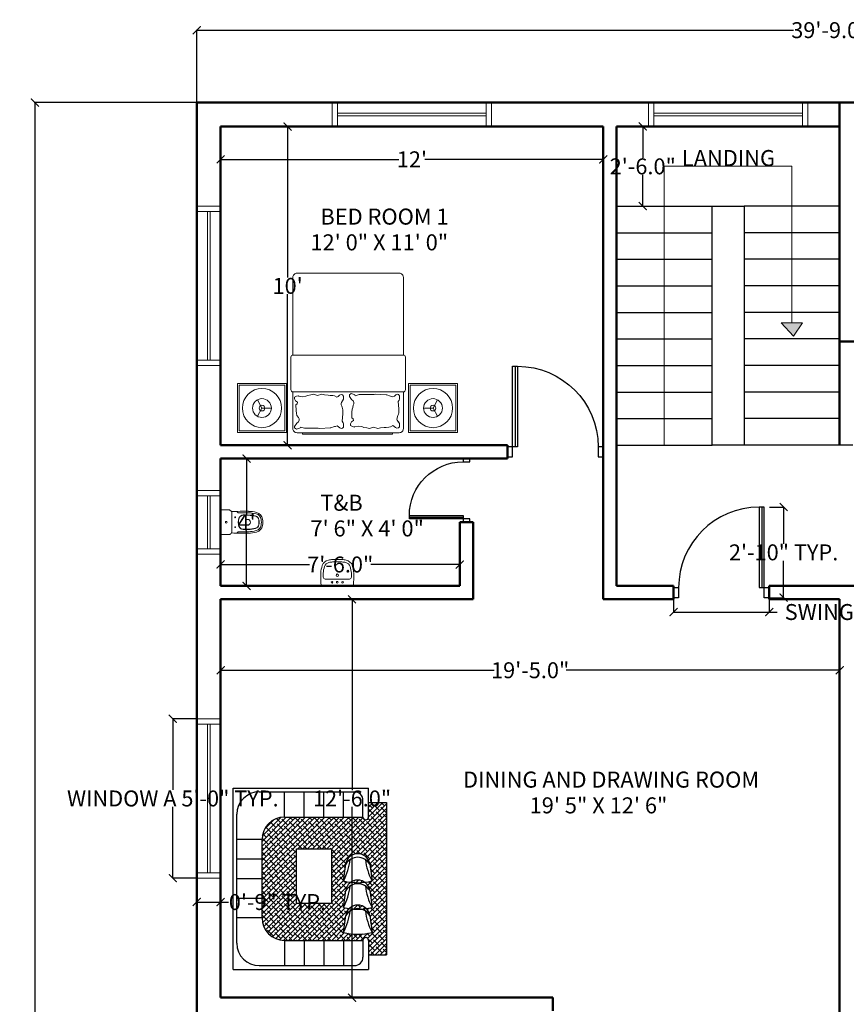
# Model space of a CAD drawing. Units: inches. Extents: x 147 to 1638, y 107 to 941.
# Tile 10 of 17: x 158 to 469, y 570 to 941. Entities that reach past the tile are written whole.
import ezdxf

# ---------------------------------------------------------------- set-up
doc = ezdxf.new("R2010")
doc.units = ezdxf.units.IN
doc.header["$MEASUREMENT"] = 0
for name, color, linetype, lineweight in [('A-ANNO-DIMS', 2, 'Continuous', 15), ('A-ANNO-SYMB', 7, 'Continuous', 18), ('A-AREA-IDEN', 7, 'Continuous', 18), ('A-Door', 150, 'Continuous', 25), ('A-FLOR-FIXT', 9, 'Continuous', 18), ('A-FLOR-STRS', 7, 'Continuous', 25), ('furniture', 50, 'Continuous', 18), ('HAT', 9, 'Continuous', 0), ('walls', 7, 'Continuous', 50), ('windows', 3, 'Continuous', 20)]:
    doc.layers.add(name, color=color, linetype=linetype, lineweight=lineweight)
for name, color, linetype in [('A-Glaz', 92, 'Continuous'), ('FUR', 42, 'Continuous'), ('NT', 1, 'Continuous'), ('Win', 152, 'Continuous')]:
    doc.layers.add(name, color=color, linetype=linetype)
doc.styles.get("Standard").update_dxf_attribs({"font": 'arial.ttf'})
doc.dimstyles.get("Standard").update_dxf_attribs({"dimtxt": 6, "dimasz": 3, "dimexe": 0.18, "dimexo": 0.0625, "dimgap": 0.09, "dimtad": 0, "dimtih": 1, "dimtoh": 1, "dimdec": 1, "dimzin": 0, "dimdsep": 46, "dimlunit": 3, "dimtxsty": 'Standard', "dimblk": 'ARCHTICK', "dimcen": 0.09, "dimadec": 0, "dimazin": 0, "dimtfac": 1, "dimtdec": 1, "dimtofl": 0, "dimtmove": 0, "dimatfit": 3, "dimfxl": 1, "dimtolj": 1, "dimtzin": 0, "dimarcsym": 0})

# ---------------------------------------------------------------- blocks, each defined once
blk = doc.blocks.new('A$C087A3AA9')
at = {"layer": 'A-Door'}
for points in [[(852.6, 94.7), (852.6, 852.6), (805.3, 852.6), (805.3, 94.7)], [(47.4, 94.7), (47.4, 0), (0, 0), (0, 94.7)], [(900, 94.7), (900, 0), (852.6, 0), (852.6, 94.7)]]:
    blk.add_lwpolyline(points, close=True, dxfattribs=at)
at = {"layer": 'A-Glaz'}
blk.add_line((828.9, 852.6), (828.9, 94.7), dxfattribs=at)
at = {"layer": 'NT'}
blk.add_arc((805.3, 94.7), 757.9, 90, 180, dxfattribs=at)
blk = doc.blocks.new('_ArchTick')
at = {"color": 0, "linetype": 'ByBlock', "const_width": 0.15}
blk.add_lwpolyline([(-0.5, -0.5), (0.5, 0.5)], dxfattribs=at)
blk = doc.blocks.new('*D3')
at = {"layer": 'A-ANNO-DIMS', "color": 0, "lineweight": -2, "transparency": 16777216}
for p, q in [((259.56, 900.72), (258.97, 900.72)), ((259.15, 900.72), (259.15, 843.87)), ((259.15, 780.72), (259.15, 837.56)), ((259.56, 780.72), (258.97, 780.72))]:
    blk.add_line(p, q, dxfattribs=at)
at = {"layer": 'Defpoints', "color": 0, "lineweight": -2, "transparency": 16777216}
for p in [(259.63, 900.72), (259.15, 780.72), (259.63, 780.72)]:
    blk.add_point(p, dxfattribs=at)
at = {"layer": 'A-ANNO-DIMS', "color": 0, "lineweight": -2, "transparency": 16777216, "xscale": 3, "yscale": 3, "zscale": 3}
for p, rotation in [((259.15, 900.72), 90), ((259.15, 780.72), 270)]:
    blk.add_blockref('_ArchTick', p, dxfattribs=dict(at, rotation=rotation))
at = {"layer": 'A-ANNO-DIMS', "color": 0, "transparency": 16777216, "insert": (259.15, 840.72), "char_height": 6, "attachment_point": 5}
blk.add_mtext("\\A1;10'", dxfattribs=at)
blk = doc.blocks.new('*D4')
at = {"layer": 'A-ANNO-DIMS', "color": 0, "lineweight": -2, "transparency": 16777216}
for p, q in [((233.94, 893.56), (233.94, 888.18)), ((377.94, 893.56), (377.94, 888.18)), ((233.94, 888.36), (301.05, 888.36)), ((377.94, 888.36), (310.84, 888.36))]:
    blk.add_line(p, q, dxfattribs=at)
at = {"layer": 'Defpoints', "color": 0, "lineweight": -2, "transparency": 16777216}
for p in [(233.94, 893.63), (377.94, 893.63), (377.94, 888.36)]:
    blk.add_point(p, dxfattribs=at)
at = {"layer": 'A-ANNO-DIMS', "color": 0, "lineweight": -2, "transparency": 16777216, "xscale": 3, "yscale": 3, "zscale": 3, "rotation": 180}
blk.add_blockref('_ArchTick', (233.94, 888.36), dxfattribs=at)
at = {"layer": 'A-ANNO-DIMS', "color": 0, "lineweight": -2, "transparency": 16777216, "xscale": 3, "yscale": 3, "zscale": 3}
blk.add_blockref('_ArchTick', (377.94, 888.36), dxfattribs=at)
at = {"layer": 'A-ANNO-DIMS', "color": 0, "transparency": 16777216, "insert": (305.94, 888.36), "char_height": 6, "attachment_point": 5}
blk.add_mtext("\\A1;12'", dxfattribs=at)
blk = doc.blocks.new('*D7')
at = {"layer": 'A-ANNO-DIMS', "color": 0, "lineweight": -2, "transparency": 16777216}
for p, q in [((389.98, 900.72), (393.01, 900.72)), ((392.83, 900.72), (392.83, 888.87)), ((392.83, 870.72), (392.83, 882.56)), ((389.98, 870.72), (393.01, 870.72))]:
    blk.add_line(p, q, dxfattribs=at)
at = {"layer": 'Defpoints', "color": 0, "lineweight": -2, "transparency": 16777216}
for p in [(389.92, 900.72), (389.92, 870.72), (392.83, 870.72)]:
    blk.add_point(p, dxfattribs=at)
at = {"layer": 'A-ANNO-DIMS', "color": 0, "lineweight": -2, "transparency": 16777216, "xscale": 3, "yscale": 3, "zscale": 3}
for p, rotation in [((392.83, 900.72), 90), ((392.83, 870.72), 270)]:
    blk.add_blockref('_ArchTick', p, dxfattribs=dict(at, rotation=rotation))
at = {"layer": 'A-ANNO-DIMS', "color": 0, "transparency": 16777216, "insert": (392.83, 885.72), "char_height": 6, "attachment_point": 5}
blk.add_mtext('\\A1;2\'-6.0"', dxfattribs=at)
blk = doc.blocks.new('*D8')
at = {"layer": 'A-ANNO-DIMS', "color": 0, "lineweight": -2, "transparency": 16777216}
for p, q in [((243.37, 775.72), (243.86, 775.72)), ((243.68, 775.72), (243.68, 754.81)), ((243.68, 727.72), (243.68, 748.63)), ((243.37, 727.72), (243.86, 727.72))]:
    blk.add_line(p, q, dxfattribs=at)
at = {"layer": 'Defpoints', "color": 0, "lineweight": -2, "transparency": 16777216}
for p in [(243.3, 775.72), (243.3, 727.72), (243.68, 727.72)]:
    blk.add_point(p, dxfattribs=at)
at = {"layer": 'A-ANNO-DIMS', "color": 0, "lineweight": -2, "transparency": 16777216, "xscale": 3, "yscale": 3, "zscale": 3}
for p, rotation in [((243.68, 775.72), 90), ((243.68, 727.72), 270)]:
    blk.add_blockref('_ArchTick', p, dxfattribs=dict(at, rotation=rotation))
at = {"layer": 'A-ANNO-DIMS', "color": 0, "transparency": 16777216, "insert": (243.68, 751.72), "char_height": 6, "attachment_point": 5}
blk.add_mtext("\\A1;4'", dxfattribs=at)
blk = doc.blocks.new('*D9')
at = {"layer": 'A-ANNO-DIMS', "color": 0, "lineweight": -2, "transparency": 16777216}
for p, q in [((233.94, 734.55), (233.94, 736)), ((233.94, 735.82), (267.41, 735.82)), ((323.94, 735.82), (290.48, 735.82)), ((323.94, 734.55), (323.94, 736))]:
    blk.add_line(p, q, dxfattribs=at)
at = {"layer": 'Defpoints', "color": 0, "lineweight": -2, "transparency": 16777216}
for p in [(233.94, 734.49), (323.94, 735.82), (323.94, 734.49)]:
    blk.add_point(p, dxfattribs=at)
at = {"layer": 'A-ANNO-DIMS', "color": 0, "lineweight": -2, "transparency": 16777216, "xscale": 3, "yscale": 3, "zscale": 3, "rotation": 180}
blk.add_blockref('_ArchTick', (233.94, 735.82), dxfattribs=at)
at = {"layer": 'A-ANNO-DIMS', "color": 0, "lineweight": -2, "transparency": 16777216, "xscale": 3, "yscale": 3, "zscale": 3}
blk.add_blockref('_ArchTick', (323.94, 735.82), dxfattribs=at)
at = {"layer": 'A-ANNO-DIMS', "color": 0, "transparency": 16777216, "insert": (278.94, 735.82), "char_height": 6, "attachment_point": 5}
blk.add_mtext('\\A1;7\'-6.0"', dxfattribs=at)
blk = doc.blocks.new('*D12')
at = {"layer": 'A-ANNO-DIMS', "color": 0, "lineweight": -2, "transparency": 16777216}
for p, q in [((278.02, 722.72), (283.58, 722.72)), ((283.4, 722.72), (283.4, 650.87)), ((283.4, 572.72), (283.4, 644.56)), ((278.02, 572.72), (283.58, 572.72))]:
    blk.add_line(p, q, dxfattribs=at)
at = {"layer": 'Defpoints', "color": 0, "lineweight": -2, "transparency": 16777216}
for p in [(277.96, 722.72), (277.96, 572.72), (283.4, 572.72)]:
    blk.add_point(p, dxfattribs=at)
at = {"layer": 'A-ANNO-DIMS', "color": 0, "lineweight": -2, "transparency": 16777216, "xscale": 3, "yscale": 3, "zscale": 3}
for p, rotation in [((283.4, 722.72), 90), ((283.4, 572.72), 270)]:
    blk.add_blockref('_ArchTick', p, dxfattribs=dict(at, rotation=rotation))
at = {"layer": 'A-ANNO-DIMS', "color": 0, "transparency": 16777216, "insert": (283.4, 647.72), "char_height": 6, "attachment_point": 5}
blk.add_mtext('\\A1;12\'-6.0"', dxfattribs=at)
blk = doc.blocks.new('*D13')
at = {"layer": 'A-ANNO-DIMS', "color": 0, "lineweight": -2, "transparency": 16777216}
for p, q in [((233.94, 696.06), (233.94, 696.18)), ((233.94, 696), (336.84, 696)), ((466.94, 696), (364.05, 696)), ((466.94, 696.06), (466.94, 696.18))]:
    blk.add_line(p, q, dxfattribs=at)
at = {"layer": 'Defpoints', "color": 0, "lineweight": -2, "transparency": 16777216}
for p in [(233.94, 696), (466.94, 696), (466.94, 696)]:
    blk.add_point(p, dxfattribs=at)
at = {"layer": 'A-ANNO-DIMS', "color": 0, "lineweight": -2, "transparency": 16777216, "xscale": 3, "yscale": 3, "zscale": 3, "rotation": 180}
blk.add_blockref('_ArchTick', (233.94, 696), dxfattribs=at)
at = {"layer": 'A-ANNO-DIMS', "color": 0, "lineweight": -2, "transparency": 16777216, "xscale": 3, "yscale": 3, "zscale": 3}
blk.add_blockref('_ArchTick', (466.94, 696), dxfattribs=at)
at = {"layer": 'A-ANNO-DIMS', "color": 0, "transparency": 16777216, "insert": (350.44, 696), "char_height": 6, "attachment_point": 5}
blk.add_mtext('\\A1;19\'-5.0"', dxfattribs=at)
blk = doc.blocks.new('*D69')
at = {"layer": 'A-ANNO-DIMS', "color": 0, "lineweight": -2, "transparency": 16777216}
for p, q in [((224.94, 909.78), (224.94, 937.18)), ((224.94, 937), (449.56, 937)), ((701.94, 937), (477.33, 937)), ((701.94, 909.78), (701.94, 937.18))]:
    blk.add_line(p, q, dxfattribs=at)
at = {"layer": 'Defpoints', "color": 0, "lineweight": -2, "transparency": 16777216}
for p in [(701.94, 937), (224.94, 909.72), (701.94, 909.72)]:
    blk.add_point(p, dxfattribs=at)
at = {"layer": 'A-ANNO-DIMS', "color": 0, "lineweight": -2, "transparency": 16777216, "xscale": 3, "yscale": 3, "zscale": 3, "rotation": 180}
blk.add_blockref('_ArchTick', (224.94, 937), dxfattribs=at)
at = {"layer": 'A-ANNO-DIMS', "color": 0, "lineweight": -2, "transparency": 16777216, "xscale": 3, "yscale": 3, "zscale": 3}
blk.add_blockref('_ArchTick', (701.94, 937), dxfattribs=at)
at = {"layer": 'A-ANNO-DIMS', "color": 0, "transparency": 16777216, "insert": (463.44, 937), "char_height": 6, "attachment_point": 5}
blk.add_mtext('\\A1;39\'-9.0"', dxfattribs=at)
blk = doc.blocks.new('*D70')
at = {"layer": 'A-ANNO-DIMS', "color": 0, "lineweight": -2, "transparency": 16777216}
for p, q in [((224.88, 909.72), (163.8, 909.72)), ((163.98, 909.72), (163.98, 558.87)), ((163.98, 201.72), (163.98, 552.56)), ((224.88, 201.72), (163.8, 201.72))]:
    blk.add_line(p, q, dxfattribs=at)
at = {"layer": 'Defpoints', "color": 0, "lineweight": -2, "transparency": 16777216}
for p in [(224.94, 909.72), (163.98, 201.72), (224.94, 201.72)]:
    blk.add_point(p, dxfattribs=at)
at = {"layer": 'A-ANNO-DIMS', "color": 0, "lineweight": -2, "transparency": 16777216, "xscale": 3, "yscale": 3, "zscale": 3}
for p, rotation in [((163.98, 909.72), 90), ((163.98, 201.72), 270)]:
    blk.add_blockref('_ArchTick', p, dxfattribs=dict(at, rotation=rotation))
at = {"layer": 'A-ANNO-DIMS', "color": 0, "transparency": 16777216, "insert": (163.98, 555.72), "char_height": 6, "attachment_point": 5}
blk.add_mtext("\\A1;59'", dxfattribs=at)
blk = doc.blocks.new('MAT-P14')
for p, q in [((-1.337, 1.348), (-1.337, 1.948)), ((-1.337, 1.948), (-0.737, 1.948)), ((-1.317, 1.928), (-0.757, 1.928)), ((-1.317, 1.368), (-1.317, 1.928)), ((-0.757, 1.368), (-0.757, 1.928)), ((-0.737, 1.348), (-0.737, 1.948)), ((0.625, 1.95), (-0.625, 1.95)), ((0.753, 1.348), (0.753, 1.948)), ((1.353, 1.948), (0.753, 1.948)), ((1.333, 1.928), (0.773, 1.928)), ((0.773, 1.368), (0.773, 1.928)), ((1.333, 1.368), (1.333, 1.928)), ((1.353, 1.348), (1.353, 1.948)), ((-1.037, 1.648), (-1.091, 1.749)), ((1.053, 1.648), (1.108, 1.749)), ((-1.037, 1.648), (-1.091, 1.547)), ((-1.037, 1.648), (-0.922, 1.648)), ((1.053, 1.648), (0.938, 1.648)), ((1.053, 1.648), (1.108, 1.547)), ((-1.337, 1.348), (-0.737, 1.348)), ((-1.317, 1.368), (-0.757, 1.368)), ((1.353, 1.348), (0.753, 1.348)), ((1.333, 1.368), (0.773, 1.368))]:
    blk.add_line(p, q)
for points in [[(-0.675, 1.45), (-0.675, 1.9, -0.414214), (-0.625, 1.95), (0.625, 1.95, -0.414214), (0.675, 1.9), (0.675, 1.45)], [(-0.675, 1, -0.414214), (-0.7, 1.025), (-0.7, 1.425, -0.414214), (-0.675, 1.45), (0.675, 1.45, -0.414214), (0.7, 1.425), (0.7, 1.025, -0.414214), (0.675, 1)], [(-0.625, 0, -0.414214), (-0.675, 0.05), (-0.675, 1), (0.675, 1), (0.675, 0.05, -0.414214), (0.625, 0)]]:
    blk.add_lwpolyline(points, format="xyb", close=True)
blk.add_lwpolyline([(-0.542, 1.95), (-0.542, 1.967), (0.558, 1.967), (0.558, 1.95)], close=True)
for points in [[(-0.614, 1.818), (-0.626, 1.838), (-0.626, 1.877), (-0.614, 1.891), (-0.596, 1.896), (-0.579, 1.886), (-0.563, 1.872), (-0.545, 1.863), (-0.516, 1.879), (-0.497, 1.882), (-0.465, 1.884), (-0.439, 1.887), (-0.395, 1.892), (-0.363, 1.9), (-0.309, 1.882), (-0.262, 1.897), (-0.23, 1.892), (-0.192, 1.884), (-0.166, 1.873), (-0.128, 1.868), (-0.082, 1.875), (-0.076, 1.88), (-0.052, 1.875), (-0.028, 1.861), (-0.028, 1.841), (-0.04, 1.817), (-0.064, 1.802), (-0.06, 1.781), (-0.043, 1.768), (-0.046, 1.697), (-0.05, 1.662), (-0.056, 1.64), (-0.062, 1.612), (-0.068, 1.596), (-0.068, 1.579), (-0.063, 1.56), (-0.039, 1.545), (-0.015, 1.505), (-0.015, 1.486), (-0.038, 1.471), (-0.075, 1.482), (-0.081, 1.487), (-0.087, 1.497), (-0.134, 1.481), (-0.304, 1.482), (-0.318, 1.482), (-0.335, 1.479), (-0.464, 1.488), (-0.467, 1.486), (-0.473, 1.486), (-0.517, 1.503), (-0.53, 1.505), (-0.548, 1.51), (-0.566, 1.501), (-0.581, 1.487), (-0.599, 1.477), (-0.617, 1.482), (-0.629, 1.497), (-0.629, 1.536), (-0.623, 1.55), (-0.611, 1.57), (-0.614, 1.614), (-0.615, 1.627), (-0.618, 1.644), (-0.619, 1.66), (-0.62, 1.675), (-0.62, 1.695), (-0.618, 1.707), (-0.614, 1.723), (-0.608, 1.739), (-0.604, 1.75), (-0.598, 1.771), (-0.596, 1.785), (-0.6, 1.798), (-0.614, 1.819)], [(0.069, 1.559), (0.057, 1.54), (0.057, 1.501), (0.069, 1.486), (0.087, 1.481), (0.105, 1.491), (0.121, 1.505), (0.139, 1.514), (0.168, 1.498), (0.187, 1.496), (0.219, 1.493), (0.244, 1.49), (0.289, 1.485), (0.321, 1.477), (0.374, 1.495), (0.422, 1.48), (0.454, 1.486), (0.492, 1.493), (0.517, 1.504), (0.555, 1.509), (0.602, 1.502), (0.608, 1.497), (0.632, 1.502), (0.656, 1.517), (0.656, 1.536), (0.644, 1.561), (0.62, 1.575), (0.624, 1.596), (0.641, 1.609), (0.637, 1.68), (0.633, 1.715), (0.628, 1.738), (0.606, 1.765), (0.6, 1.781), (0.6, 1.798), (0.605, 1.817), (0.629, 1.832), (0.654, 1.872), (0.654, 1.892), (0.63, 1.906), (0.593, 1.895), (0.587, 1.891), (0.581, 1.881), (0.534, 1.896), (0.379, 1.896), (0.366, 1.896), (0.348, 1.898), (0.22, 1.89), (0.216, 1.891), (0.21, 1.891), (0.167, 1.875), (0.154, 1.872), (0.136, 1.867), (0.118, 1.876), (0.102, 1.89), (0.085, 1.9), (0.067, 1.895), (0.055, 1.881), (0.055, 1.842), (0.061, 1.827), (0.073, 1.807), (0.07, 1.764), (0.069, 1.75), (0.066, 1.733), (0.065, 1.718), (0.063, 1.703), (0.063, 1.682), (0.066, 1.67), (0.07, 1.655), (0.075, 1.638), (0.079, 1.627), (0.086, 1.607), (0.087, 1.592), (0.083, 1.579), (0.07, 1.559)]]:
    blk.add_lwpolyline(points)
for centre, radius in [((-1.037, 1.648), 0.24), ((1.053, 1.648), 0.24), ((-1.037, 1.648), 0.115), ((1.053, 1.648), 0.115), ((-1.037, 1.648), 0.035), ((1.053, 1.648), 0.035)]:
    blk.add_circle(centre, radius)
blk = doc.blocks.new('2SAINDA')
at = {"color": 0, "linetype": 'ByBlock'}
for p, q in [((0, 0.188), (0, -0.188)), ((0.018, 0.2), (0.141, 0.2)), ((0.157, 0.192), (0.162, 0.188)), ((0.18, -0.164), (0.18, 0.164)), ((0.279, 0.159), (0.261, 0.176)), ((0.437, 0.047), (0.424, 0.047)), ((0.279, -0.159), (0.261, -0.176)), ((0.437, -0.047), (0.424, -0.047)), ((0.018, -0.2), (0.141, -0.2)), ((0.157, -0.192), (0.162, -0.188))]:
    blk.add_line(p, q, dxfattribs=at)
for centre, radius in [((0.09, 0), 0.0135), ((0.09, 0), 0.0135), ((0.236, 0.08), 0.0075), ((0.236, -0.08), 0.0075)]:
    blk.add_circle(centre, radius, dxfattribs=at)
for centre, radius, start, end in [((0.018, 0.18), 0.02, 90, 155.6901), ((0.141, 0.181), 0.019, 34.9372, 90), ((0.155, 0.164), 0.025, 23.3776, 73.7848), ((0.383, -5.322), 5.5, 89.2905, 92.1362), ((0.155, 0.164), 0.025, 360, 23.3776), ((0.444, -0.373), 0.55, 75.4605, 89.2905), ((0.293, 0.173), 0.02, 225, 270.9364), ((0.485, 0), 0.2, 160.016, 199.984), ((0.485, 0), 0.196, 160.016, 199.984), ((0.383, -5.322), 5.476, 89.2905, 90.9364), ((0.368, 0.043), 0.075, 90.1648, 160.016), ((0.368, 0.043), 0.071, 90.1648, 160.016), ((0.383, -5.322), 5.44, 89.2905, 90.1648), ((0.383, -5.322), 5.436, 89.2905, 90.1648), ((0.582, 0), 0.18, 170.2849, 189.7151), ((0.424, 0.027), 0.02, 90, 170.2849), ((0.437, 0), 0.047, 0, 90), ((0.437, 0), 0.047, 270, 0), ((0.444, -0.373), 0.49, 75.4605, 89.2905), ((0.444, -0.373), 0.486, 75.4605, 89.2905), ((0.444, -0.373), 0.526, 75.4605, 89.2905), ((0.549, 0.03), 0.07, 8.8162, 75.4605), ((0.549, 0.03), 0.074, 8.8162, 75.4605), ((0.549, 0.03), 0.11, 8.8162, 75.4605), ((0.549, 0.03), 0.134, 8.8162, 75.4605), ((0.355, 0), 0.266, 351.1838, 8.8162), ((0.355, 0), 0.27, 351.1838, 8.8162), ((0.355, 0), 0.306, 351.1838, 8.8162), ((0.355, 0), 0.33, 351.1838, 8.8162), ((0.293, -0.173), 0.02, 89.0636, 135), ((0.383, 5.322), 5.476, 269.0636, 270.7095), ((0.368, -0.043), 0.075, 199.984, 269.8352), ((0.368, -0.043), 0.071, 199.984, 269.8352), ((0.383, 5.322), 5.436, 269.8352, 270.7095), ((0.383, 5.322), 5.44, 269.8352, 270.7095), ((0.424, -0.027), 0.02, 189.7151, 270), ((0.444, 0.373), 0.486, 270.7095, 284.5395), ((0.444, 0.373), 0.49, 270.7095, 284.5395), ((0.444, 0.373), 0.526, 270.7095, 284.5395), ((0.444, 0.373), 0.55, 270.7095, 284.5395), ((0.549, -0.03), 0.07, 284.5395, 351.1838), ((0.549, -0.03), 0.074, 284.5395, 351.1838), ((0.549, -0.03), 0.11, 284.5395, 351.1838), ((0.549, -0.03), 0.134, 284.5395, 351.1838), ((0.018, -0.18), 0.02, 204.3099, 270), ((0.141, -0.181), 0.019, 270, 325.0628), ((0.155, -0.164), 0.025, 286.2152, 336.6224), ((0.155, -0.164), 0.025, 336.6224, 0), ((0.383, 5.322), 5.5, 267.8638, 270.7095)]:
    blk.add_arc(centre, radius, start, end, dxfattribs=at)
blk = doc.blocks.new('2SALADA2')
at = {"color": 0}
for p, q in [((-0.296, 0), (0.296, 0)), ((0.207, -0.13), (-0.207, -0.13))]:
    blk.add_line(p, q, dxfattribs=at)
for centre, radius in [((-0.1, -0.07), 0.015), ((0, -0.205), 0.023), ((0, -0.07), 0.0175), ((0.1, -0.07), 0.015)]:
    blk.add_circle(centre, radius, dxfattribs=at)
for centre, radius, start, end in [((-0.296, -0.01), 0.01, 90, 173.6262), ((0.296, -0.01), 0.01, 6.3738, 90), ((1.185, -0.175), 1.5, 173.6262, 182.693), ((1.186, -0.221), 1.454, 178.0234, 180.898), ((-0.227, -0.171), 0.04, 95.5937, 179.6995), ((-0.207, -0.38), 0.25, 90, 95.5937), ((0.207, -0.38), 0.25, 84.4063, 90), ((0.227, -0.171), 0.04, 0.3005, 84.4063), ((-1.186, -0.221), 1.454, 359.102, 1.9766), ((-1.185, -0.175), 1.5, 357.307, 6.3738), ((0.186, -0.222), 0.5, 182.693, 199.3406), ((0.186, -0.222), 0.454, 182.693, 199.3406), ((-0.135, -0.335), 0.114, 199.3406, 257.4429), ((0.135, -0.335), 0.114, 282.5571, 340.6594), ((-0.186, -0.222), 0.454, 340.6594, 357.307), ((-0.186, -0.222), 0.5, 340.6594, 357.307), ((-0.135, -0.335), 0.16, 199.3406, 257.4429), ((-0.061, -0.003), 0.5, 257.4429, 266.4982), ((-0.061, -0.003), 0.454, 257.4429, 266.4982), ((0, 0.995), 1.5, 266.4982, 273.5018), ((0, 0.995), 1.454, 266.4982, 273.5018), ((0.061, -0.003), 0.454, 273.5018, 282.5571), ((0.061, -0.003), 0.5, 273.5018, 282.5571), ((0.135, -0.335), 0.16, 282.5571, 340.6594)]:
    blk.add_arc(centre, radius, start, end, dxfattribs=at)
blk = doc.blocks.new('CHAIR1')
for p, q in [((-393, -750), (-329, -287)), ((329, -286), (394, -750))]:
    blk.add_line(p, q)
for centre, radius, start, end in [((0, -332), 332, 7.9072, 172.1612), ((-1856, 27), 1657, 332.0394, 353.4161), ((0, -483), 383, 30.9021, 149.1663), ((1857, 27), 1657, 186.5839, 207.9606), ((0, 770), 1570, 255.502, 284.498)]:
    blk.add_arc(centre, radius, start, end)
blk = doc.blocks.new('A$C1CFC4E3A')
at = {"layer": 'HAT'}
h = blk.add_hatch(dxfattribs=at)
h.set_pattern_fill('ANSI38,_O', color=256, scale=0.664121)
h.set_pattern_definition([(45, (6.13299, -18.48134), (-0.05870057, 0.05870057), []), (135, (6.13299, -18.48134), (-0.1761017, 0.05870057), [0.2075378, -0.1245227])])
h.paths.add_polyline_path([(0, 3.705), (-0.438, 3.705), (-0.438, 3.353, -1), (-0.573, 3.353), (-2.482, 3.353, 0.414214), (-3.028, 2.807), (-3.028, 0.898, 0.414214), (-2.482, 0.352), (-0.573, 0.352, -1), (-0.438, 0.352), (-0.438, 0), (0, 0)])
h.paths.add_polyline_path([(-1.342, 1.248), (-2.191, 1.248), (-2.191, 2.58), (-1.342, 2.58)], flags=16)
h.paths.add_polyline_path([(-0.409, 1.566), (-0.352, 1.156, -0.127199), (-1.048, 1.156), (-0.992, 1.566, -0.871235)], flags=16)
h.paths.add_polyline_path([(-0.409, 0.959), (-0.352, 0.548, -0.127199), (-1.048, 0.548), (-0.992, 0.958, -0.871235)], flags=16)
h.paths.add_polyline_path([(-0.992, 2.209, -0.871235), (-0.409, 2.21), (-0.352, 1.799, -0.127199), (-1.048, 1.799)], flags=16)
at = {"layer": 'FUR'}
for p, q in [((-3.732, 4.057), (-0.438, 4.057)), ((-3.732, -0.352), (-3.732, 4.057)), ((-3.096, 3.967), (-0.777, 3.967)), ((-2.482, 3.353), (-2.482, 3.967)), ((-2.005, 3.353), (-2.005, 3.967)), ((-1.528, 3.353), (-1.528, 3.967)), ((-1.05, 3.353), (-1.05, 3.967)), ((-0.438, 3.353), (-0.438, 4.057)), ((-0.573, 3.353), (-0.573, 3.762)), ((-3.642, 0.284), (-3.642, 3.421)), ((-2.482, 3.353), (-0.573, 3.353)), ((-3.028, 2.807), (-3.642, 2.807)), ((-3.028, 2.33), (-3.642, 2.33)), ((-3.028, 1.852), (-3.642, 1.852)), ((-3.028, 1.375), (-3.642, 1.375)), ((-3.028, 0.898), (-3.642, 0.898)), ((-2.482, 0.352), (-0.573, 0.352)), ((-2.482, 0.352), (-2.482, -0.262)), ((-2.005, 0.352), (-2.005, -0.262)), ((-1.528, 0.352), (-1.528, -0.262)), ((-1.05, 0.352), (-1.05, -0.262)), ((-0.573, 0.352), (-0.573, -0.057)), ((-0.438, 0.352), (-0.438, -0.352)), ((-3.732, -0.352), (-0.438, -0.352)), ((-3.096, -0.262), (-0.777, -0.262))]:
    blk.add_line(p, q, dxfattribs=at)
for centre, radius, start, end in [((-3.096, 3.421), 0.546, 90, 180), ((-0.777, 3.762), 0.205, 0, 90), ((-2.482, 2.807), 0.546, 90, 180), ((-0.505, 3.353), 0.0675, 180, 0), ((-2.482, 0.898), 0.546, 180, 270), ((-3.096, 0.284), 0.546, 180, 270), ((-0.505, 0.352), 0.0675, 0, 180), ((-0.777, -0.057), 0.205, 270, 0)]:
    blk.add_arc(centre, radius, start, end, dxfattribs=at)
at = {"layer": 'Win'}
for p, q in [((-0.438, 3.705), (0, 3.705)), ((0, 3.705), (0, 0)), ((-3.028, 0.898), (-3.028, 2.807)), ((-0.438, 0), (0, 0))]:
    blk.add_line(p, q, dxfattribs=at)
blk.add_lwpolyline([(-2.191, 2.58), (-1.342, 2.58), (-1.342, 1.248), (-2.191, 1.248)], close=True, dxfattribs=at)
at = {"layer": 'FUR', "xscale": 0.0008854948152227, "yscale": 0.0008854948152227, "zscale": 0.0008854948152227}
for p in [(-0.7, 2.463), (-0.7, 1.82), (-0.7, 1.212)]:
    blk.add_blockref('CHAIR1', p, dxfattribs=at)
blk = doc.blocks.new('WIN-60IN')
for p, q in [((60, 9), (0, 9)), ((0, 9), (0, 0)), ((2, 9), (2, 0)), ((58, 0), (58, 9)), ((60, 0), (60, 9)), ((2, 5), (58, 5)), ((2, 4), (58, 4)), ((0, 0), (60, 0))]:
    blk.add_line(p, q)
blk = doc.blocks.new('WIN-24IN')
for p, q in [((9, 24), (0, 24)), ((0, 24), (0, 0)), ((9, 0), (9, 24)), ((9, 22), (0, 22)), ((4, 2), (4, 22)), ((5, 2), (5, 22)), ((0, 2), (9, 2)), ((0, 0), (9, 0))]:
    blk.add_line(p, q)
blk = doc.blocks.new('STAIR-RETURN-FLIGHTS')
for p, q in [((0, 90), (36, 90)), ((36, 0), (36, 90)), ((36, 90), (48, 90)), ((84, 90), (48, 90)), ((48, 90), (48, 0)), ((0, 80), (36, 80)), ((84, 80), (48, 80)), ((0, 70), (36, 70)), ((84, 70), (48, 70)), ((0, 60), (36, 60)), ((84, 60), (48, 60)), ((0, 50), (36, 50)), ((84, 50), (48, 50)), ((0, 40), (36, 40)), ((84, 40), (48, 40)), ((0, 30), (36, 30)), ((84, 30), (48, 30)), ((0, 20), (36, 20)), ((84, 20), (48, 20)), ((0, 10), (36, 10)), ((84, 10), (48, 10)), ((0, 0), (36, 0)), ((48, 0), (36, 0)), ((89, 0), (48, 0))]:
    blk.add_line(p, q)
blk = doc.blocks.new('STAIR-DIRECTION-RETURN')
h = blk.add_hatch(color=256)
h.dxf.hatch_style = 1
h.paths.add_polyline_path([(52, 46.08), (48, 46.08), (44, 46.08), (48.61, 41.07)])
for p, q in [((0, 0), (0, 105.11)), ((0, 105.11), (48, 105.11)), ((48, 105.11), (48, 46.08)), ((48, 46.08), (44, 46.08)), ((48.61, 41.07), (44, 46.08)), ((48, 46.08), (52, 46.08)), ((52, 46.08), (48.61, 41.07))]:
    blk.add_line(p, q)
blk = doc.blocks.new('*D100')
at = {"layer": 'A-ANNO-DIMS', "color": 0, "lineweight": -2, "transparency": 16777216}
for p, q in [((404.44, 723.26), (404.44, 717.74)), ((440.44, 723.26), (440.44, 717.74)), ((404.44, 717.92), (440.44, 717.92)), ((440.44, 717.92), (443.44, 717.92))]:
    blk.add_line(p, q, dxfattribs=at)
at = {"layer": 'Defpoints', "color": 0, "lineweight": -2, "transparency": 16777216}
for p in [(404.44, 723.32), (440.44, 723.32), (440.44, 717.92)]:
    blk.add_point(p, dxfattribs=at)
at = {"layer": 'A-ANNO-DIMS', "color": 0, "lineweight": -2, "transparency": 16777216, "xscale": 3, "yscale": 3, "zscale": 3, "rotation": 180}
blk.add_blockref('_ArchTick', (404.44, 717.92), dxfattribs=at)
at = {"layer": 'A-ANNO-DIMS', "color": 0, "lineweight": -2, "transparency": 16777216, "xscale": 3, "yscale": 3, "zscale": 3}
blk.add_blockref('_ArchTick', (440.44, 717.92), dxfattribs=at)
at = {"layer": 'A-ANNO-DIMS', "color": 0, "transparency": 16777216, "insert": (490.91, 717.92), "char_height": 6, "attachment_point": 5}
blk.add_mtext('\\A1;SWING DOOR 3\'-0" TYP.', dxfattribs=at)
blk = doc.blocks.new('*D101')
at = {"layer": 'A-ANNO-DIMS', "color": 0, "lineweight": -2, "transparency": 16777216}
for p, q in [((440.51, 757.43), (446.02, 757.43)), ((445.84, 757.43), (445.84, 743.53)), ((445.84, 723.32), (445.84, 737.22)), ((440.51, 723.32), (446.02, 723.32))]:
    blk.add_line(p, q, dxfattribs=at)
at = {"layer": 'Defpoints', "color": 0, "lineweight": -2, "transparency": 16777216}
for p in [(440.44, 757.43), (445.84, 757.43), (440.44, 723.32)]:
    blk.add_point(p, dxfattribs=at)
at = {"layer": 'A-ANNO-DIMS', "color": 0, "lineweight": -2, "transparency": 16777216, "xscale": 3, "yscale": 3, "zscale": 3}
for p, rotation in [((445.84, 757.43), 90), ((445.84, 723.32), 270)]:
    blk.add_blockref('_ArchTick', p, dxfattribs=dict(at, rotation=rotation))
at = {"layer": 'A-ANNO-DIMS', "color": 0, "transparency": 16777216, "insert": (445.84, 740.38), "char_height": 6, "attachment_point": 5}
blk.add_mtext('\\A1;2\'-10" TYP.', dxfattribs=at)
blk = doc.blocks.new('*D102')
at = {"layer": 'A-ANNO-DIMS', "color": 0, "lineweight": -2, "transparency": 16777216}
for p, q in [((224.88, 677.72), (215.76, 677.72)), ((215.94, 677.72), (215.94, 650.91)), ((215.94, 617.72), (215.94, 644.52)), ((224.88, 617.72), (215.76, 617.72))]:
    blk.add_line(p, q, dxfattribs=at)
at = {"layer": 'Defpoints', "color": 0, "lineweight": -2, "transparency": 16777216}
for p in [(224.94, 677.72), (215.94, 617.72), (224.94, 617.72)]:
    blk.add_point(p, dxfattribs=at)
at = {"layer": 'A-ANNO-DIMS', "color": 0, "lineweight": -2, "transparency": 16777216, "xscale": 3, "yscale": 3, "zscale": 3}
for p, rotation in [((215.94, 677.72), 90), ((215.94, 617.72), 270)]:
    blk.add_blockref('_ArchTick', p, dxfattribs=dict(at, rotation=rotation))
at = {"layer": 'A-ANNO-DIMS', "color": 0, "transparency": 16777216, "insert": (215.94, 647.72), "char_height": 6, "attachment_point": 5}
blk.add_mtext('\\A1;WINDOW A 5\'-0" TYP.', dxfattribs=at)
blk = doc.blocks.new('*D103')
at = {"layer": 'A-ANNO-DIMS', "color": 0, "lineweight": -2, "transparency": 16777216}
for p, q in [((224.94, 617.66), (224.94, 608.54)), ((233.94, 617.66), (233.94, 608.54)), ((224.94, 608.72), (233.94, 608.72)), ((233.94, 608.72), (236.94, 608.72))]:
    blk.add_line(p, q, dxfattribs=at)
at = {"layer": 'Defpoints', "color": 0, "lineweight": -2, "transparency": 16777216}
for p in [(224.94, 617.72), (233.94, 617.72), (233.94, 608.72)]:
    blk.add_point(p, dxfattribs=at)
at = {"layer": 'A-ANNO-DIMS', "color": 0, "lineweight": -2, "transparency": 16777216, "xscale": 3, "yscale": 3, "zscale": 3, "rotation": 180}
blk.add_blockref('_ArchTick', (224.94, 608.72), dxfattribs=at)
at = {"layer": 'A-ANNO-DIMS', "color": 0, "lineweight": -2, "transparency": 16777216, "xscale": 3, "yscale": 3, "zscale": 3}
blk.add_blockref('_ArchTick', (233.94, 608.72), dxfattribs=at)
at = {"layer": 'A-ANNO-DIMS', "color": 0, "transparency": 16777216, "insert": (255.32, 608.72), "char_height": 6, "attachment_point": 5}
blk.add_mtext('\\A1;0\'-9" TYP.', dxfattribs=at)
blk = doc.blocks.new('*D115')
at = {"layer": 'A-ANNO-DIMS', "color": 0, "lineweight": -2, "transparency": 16777216}
for p, q in [((376.42, 560.68), (373.42, 560.68)), ((376.42, 547.98), (376.42, 560.86)), ((425.95, 560.68), (376.42, 560.68)), ((425.95, 547.98), (425.95, 560.86))]:
    blk.add_line(p, q, dxfattribs=at)
at = {"layer": 'Defpoints', "color": 0, "lineweight": -2, "transparency": 16777216}
for p in [(376.42, 560.68), (376.42, 547.91), (425.95, 547.91)]:
    blk.add_point(p, dxfattribs=at)
at = {"layer": 'A-ANNO-DIMS', "color": 0, "lineweight": -2, "transparency": 16777216, "xscale": 3, "yscale": 3, "zscale": 3, "rotation": 180}
blk.add_blockref('_ArchTick', (376.42, 560.68), dxfattribs=at)
at = {"layer": 'A-ANNO-DIMS', "color": 0, "lineweight": -2, "transparency": 16777216, "xscale": 3, "yscale": 3, "zscale": 3}
blk.add_blockref('_ArchTick', (425.95, 560.68), dxfattribs=at)
at = {"layer": 'A-ANNO-DIMS', "color": 0, "transparency": 16777216, "insert": (347.93, 560.68), "char_height": 6, "attachment_point": 5}
blk.add_mtext('\\A1;4\'-1 1/2" TYP.', dxfattribs=at)

msp = doc.modelspace()

# ---------------------------------------------------------------- linework, layer by layer
at = {"layer": 'walls'}
for p, q in [((224.94, 909.72), (224.94, 201.72)), ((224.94, 909.72), (701.94, 909.72)), ((466.94, 909.72), (466.94, 780.72)), ((233.94, 900.72), (377.94, 900.72)), ((233.94, 900.72), (233.94, 780.72)), ((377.94, 900.72), (377.94, 780.72)), ((382.94, 900.72), (382.94, 727.72)), ((382.94, 900.72), (466.94, 900.72)), ((466.94, 819.72), (495.94, 819.72)), ((233.94, 780.72), (341.94, 780.72)), ((341.94, 780.72), (341.94, 775.72)), ((377.94, 780.72), (377.94, 775.72)), ((233.94, 775.72), (323.94, 775.72)), ((233.94, 775.72), (233.94, 727.72)), ((323.94, 775.72), (328.94, 775.72)), ((328.94, 775.72), (341.94, 775.72)), ((377.94, 775.72), (377.94, 722.72)), ((323.94, 751.72), (323.94, 727.72)), ((323.94, 751.72), (328.94, 751.72)), ((328.94, 751.72), (328.94, 722.72)), ((233.94, 727.72), (323.94, 727.72)), ((382.94, 727.72), (404.44, 727.72)), ((404.44, 722.72), (404.44, 727.72)), ((440.44, 722.72), (440.44, 727.72)), ((440.44, 727.72), (492.44, 727.72)), ((233.94, 722.72), (328.94, 722.72)), ((233.94, 722.72), (233.94, 572.72)), ((377.94, 722.72), (404.44, 722.72)), ((440.44, 722.72), (466.94, 722.72)), ((466.94, 722.72), (466.94, 400.72)), ((233.94, 572.72), (358.94, 572.72)), ((358.94, 572.72), (358.94, 567.72))]:
    msp.add_line(p, q, dxfattribs=at)

# ---------------------------------------------------------------- block references
at = {"layer": 'A-ANNO-SYMB'}
msp.add_blockref('STAIR-DIRECTION-RETURN', (400.94, 780.72), dxfattribs=at)
at = {"layer": 'A-Door', "yscale": 0.0400000000000001, "zscale": 0.0400000000000001}
for p, xscale in [((377.94, 776.32), -0.0400000000000001), ((404.44, 723.32), 0.0400000000000001)]:
    msp.add_blockref('A$C087A3AA9', p, dxfattribs=dict(at, xscale=xscale))
at = {"layer": 'A-Door', "xscale": -0.0266666667542921, "yscale": 0.0266666667542921, "zscale": 0.0266666667542921, "rotation": 90}
msp.add_blockref('A$C087A3AA9', (327.71, 775.72), dxfattribs=at)
at = {"layer": 'A-FLOR-FIXT', "xscale": 23.19012112898009, "yscale": 23.19012112898009, "zscale": 23.19012112898009}
msp.add_blockref('2SAINDA', (233.94, 751.72), dxfattribs=at)
at = {"layer": 'A-FLOR-FIXT', "xscale": 19.81841434140962, "yscale": 19.81841434140962, "zscale": 19.81841434140962, "rotation": 180}
msp.add_blockref('2SALADA2', (277.84, 727.72), dxfattribs=at)
at = {"layer": 'A-FLOR-STRS'}
msp.add_blockref('STAIR-RETURN-FLIGHTS', (382.94, 780.72), dxfattribs=at)
at = {"layer": 'furniture', "xscale": 30.80045642108221, "yscale": 30.80045642108221, "zscale": 30.80045642108221, "rotation": 180}
msp.add_blockref('MAT-P14', (281.93, 845.48), dxfattribs=at)
at = {"layer": 'furniture', "xscale": 15.47145176415956, "yscale": 15.47145176415956, "zscale": 15.47145176415956}
msp.add_blockref('A$C1CFC4E3A', (296.37, 588.83), dxfattribs=at)
at = {"layer": 'windows'}
for p, rotation in [((335.94, 909.72), 180), ((224.94, 870.72), 270.0000000000007), ((224.94, 677.72), 270.0000000000007)]:
    msp.add_blockref('WIN-60IN', p, dxfattribs=dict(at, rotation=rotation))
for name, p in [('WIN-60IN', (394.94, 900.72)), ('WIN-24IN', (224.94, 739.72))]:
    msp.add_blockref(name, p, dxfattribs=at)

# ---------------------------------------------------------------- texts
at = {"layer": 'A-AREA-IDEN'}
for s, height, p in [('LANDING', 6.031, (407.53, 885.83)), ('BED ROOM 1', 6.031, (271.48, 863.78)), ('  12\' 0" X 11\' 0"', 6.0306, (264.04, 854.09)), ('T&B', 6.031, (271.48, 756.05)), ('  7\' 6" X 4\' 0"', 6.0306, (264.04, 746.37)), ('DINING AND DRAWING ROOM', 6.0306, (325.17, 651.8)), ('19\' 5" X 12\' 6"', 6.0306, (350.24, 642.11))]:
    msp.add_text(s, height=height, dxfattribs=at).set_placement(p)

# ---------------------------------------------------------------- dimensions: what is measured, and where the dimension line sits
at = {"layer": 'A-ANNO-DIMS'}
for base, p1, p2, picture, middle in [((701.94, 937), (224.94, 909.72), (701.94, 909.72), '*D69', (463.44, 937)), ((377.94, 888.36), (233.94, 893.63), (377.94, 893.63), '*D4', (305.94, 888.36)), ((323.94, 735.82), (233.94, 734.49), (323.94, 734.49), '*D9', (278.94, 735.82)), ((466.94, 696), (233.94, 696), (466.94, 696), '*D13', (350.44, 696))]:
    dim = msp.add_linear_dim(base=base, p1=p1, p2=p2, dimstyle='Standard', override={"dimclrd": 0, "dimclre": 0, "dimclrt": 0}, dxfattribs=at)
    dim.commit()
    dim.dimension.update_dxf_attribs({"geometry": picture, "text_midpoint": middle})
for base, p1, p2, picture, middle in [((163.98, 201.72), (224.94, 909.72), (224.94, 201.72), '*D70', (163.98, 555.72)), ((259.15, 780.72), (259.63, 900.72), (259.63, 780.72), '*D3', (259.15, 840.72)), ((392.83, 870.72), (389.92, 900.72), (389.92, 870.72), '*D7', (392.83, 885.72)), ((243.68, 727.72), (243.3, 775.72), (243.3, 727.72), '*D8', (243.68, 751.72)), ((283.4, 572.72), (277.96, 722.72), (277.96, 572.72), '*D12', (283.4, 647.72))]:
    dim = msp.add_linear_dim(base=base, p1=p1, p2=p2, angle=90, dimstyle='Standard', override={"dimclrd": 0, "dimclre": 0, "dimclrt": 0}, dxfattribs=at)
    dim.commit()
    dim.dimension.update_dxf_attribs({"geometry": picture, "text_midpoint": middle})
for base, p1, p2, angle, text, picture, middle in [((445.84, 757.43), (440.44, 723.32), (440.44, 757.43), 90, '<> TYP.', '*D101', (445.84, 740.38)), ((215.94, 617.72), (224.94, 677.72), (224.94, 617.72), 270, 'WINDOW A <> TYP.', '*D102', (215.94, 647.72)), ((233.94, 608.72), (224.94, 617.72), (233.94, 617.72), 0, '<> TYP.', '*D103', (255.32, 608.72)), ((376.42, 560.68), (425.95, 547.91), (376.42, 547.91), 180, '<> TYP.', '*D115', (347.93, 560.68))]:
    dim = msp.add_linear_dim(base=base, p1=p1, p2=p2, angle=angle, text=text, dimstyle='Standard', override={"dimdec": 1, "dimlfac": 1, "dimrnd": 0, "dimzin": 1, "dimdsep": 46, "dimlunit": 4, "dimfrac": 2}, dxfattribs=at)
    dim.commit()
    dim.dimension.update_dxf_attribs({"geometry": picture, "text_midpoint": middle})
dim = msp.add_linear_dim(base=(440.44, 717.92), p1=(404.44, 723.32), p2=(440.44, 723.32), text='SWING DOOR <> TYP.', dimstyle='Standard', override={"dimdec": 1, "dimlfac": 1, "dimrnd": 0, "dimzin": 1, "dimdsep": 46, "dimlunit": 4, "dimfrac": 2}, dxfattribs=at)
dim.commit()
dim.dimension.update_dxf_attribs({"geometry": '*D100', "text_midpoint": (490.91, 717.92)})

doc.saveas('drawing.dxf')
